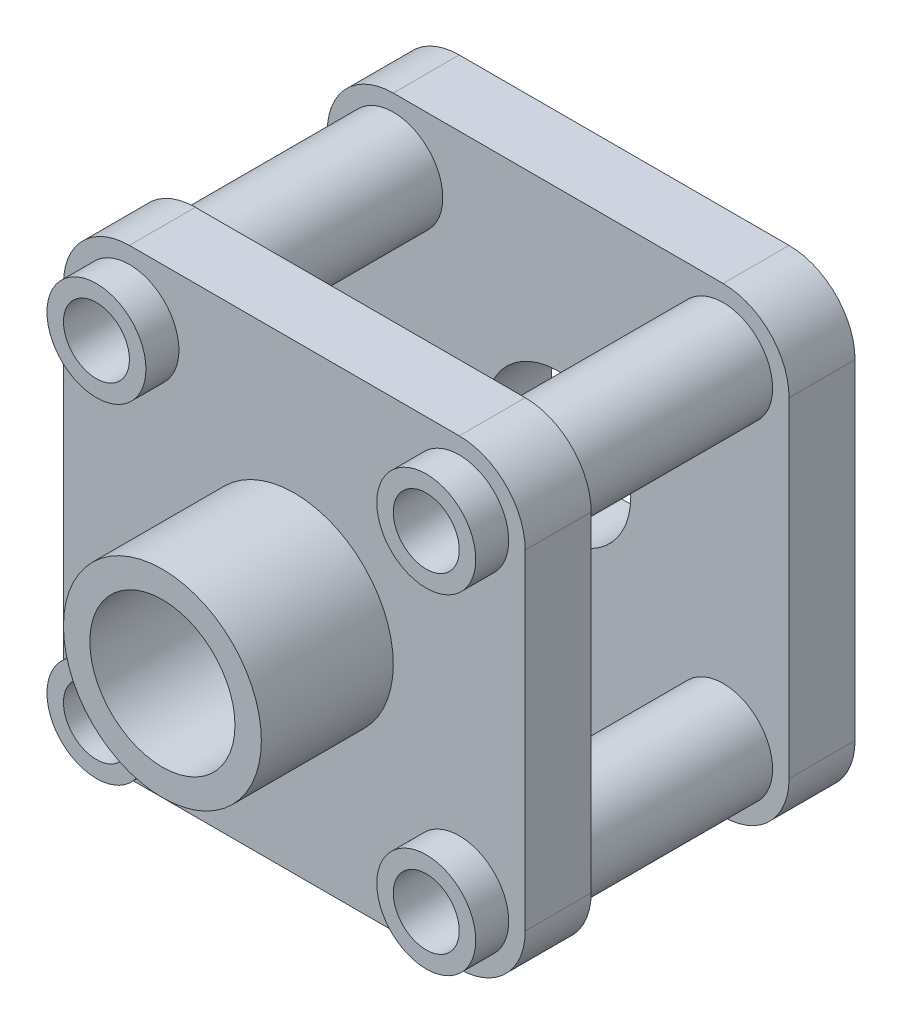
ISO-10303-21;
HEADER;
FILE_DESCRIPTION(('STEP AP214'),'2;1');
FILE_NAME('part.step','',(''),(''),'','','');
FILE_SCHEMA(('AUTOMOTIVE_DESIGN { 1 0 10303 214 1 1 1 1 }'));
ENDSEC;
DATA;
#1=APPLICATION_CONTEXT('core data for automotive mechanical design processes');
#2=APPLICATION_PROTOCOL_DEFINITION('international standard','automotive_design',2000,#1);
#3=PRODUCT_CONTEXT('',#1,'mechanical');
#4=PRODUCT('Part','Part','',(#3));
#5=PRODUCT_RELATED_PRODUCT_CATEGORY('part','',(#4));
#6=PRODUCT_DEFINITION_FORMATION('','',#4);
#7=PRODUCT_DEFINITION_CONTEXT('part definition',#1,'design');
#8=PRODUCT_DEFINITION('design','',#6,#7);
#9=PRODUCT_DEFINITION_SHAPE('','',#8);
#10=(LENGTH_UNIT() NAMED_UNIT(*) SI_UNIT(.MILLI.,.METRE.));
#11=(NAMED_UNIT(*) PLANE_ANGLE_UNIT() SI_UNIT($,.RADIAN.));
#12=(NAMED_UNIT(*) SI_UNIT($,.STERADIAN.) SOLID_ANGLE_UNIT());
#13=UNCERTAINTY_MEASURE_WITH_UNIT(LENGTH_MEASURE(1.E-05),#10,'distance_accuracy_value','');
#14=(GEOMETRIC_REPRESENTATION_CONTEXT(3) GLOBAL_UNCERTAINTY_ASSIGNED_CONTEXT((#13)) GLOBAL_UNIT_ASSIGNED_CONTEXT((#10,
#11,#12)) REPRESENTATION_CONTEXT('',''));
#15=CARTESIAN_POINT('',(0.,0.,0.));
#16=DIRECTION('',(0.,0.,1.));
#17=DIRECTION('',(1.,0.,0.));
#18=AXIS2_PLACEMENT_3D('',#15,#16,#17);
#19=CARTESIAN_POINT('',(0.,70.,10.));
#20=DIRECTION('',(1.,0.,0.));
#21=DIRECTION('',(0.,0.,-1.));
#22=AXIS2_PLACEMENT_3D('',#19,#20,#21);
#23=PLANE('',#22);
#24=DIRECTION('',(0.,-1.,0.));
#25=VECTOR('',#24,1.);
#26=CARTESIAN_POINT('',(0.,70.,0.));
#27=LINE('',#26,#25);
#28=CARTESIAN_POINT('',(0.,60.,0.));
#29=VERTEX_POINT('',#28);
#30=CARTESIAN_POINT('',(0.,10.,0.));
#31=VERTEX_POINT('',#30);
#32=EDGE_CURVE('E216',#29,#31,#27,.T.);
#33=ORIENTED_EDGE('',*,*,#32,.T.);
#34=DIRECTION('',(0.,0.,-1.));
#35=VECTOR('',#34,1.);
#36=CARTESIAN_POINT('',(0.,10.,10.));
#37=LINE('',#36,#35);
#38=CARTESIAN_POINT('',(0.,10.,10.));
#39=VERTEX_POINT('',#38);
#40=EDGE_CURVE('E11',#31,#39,#37,.F.);
#41=ORIENTED_EDGE('',*,*,#40,.T.);
#42=DIRECTION('',(0.,-1.,0.));
#43=VECTOR('',#42,1.);
#44=CARTESIAN_POINT('',(0.,70.,10.));
#45=LINE('',#44,#43);
#46=CARTESIAN_POINT('',(0.,60.,10.));
#47=VERTEX_POINT('',#46);
#48=EDGE_CURVE('E217',#47,#39,#45,.T.);
#49=ORIENTED_EDGE('',*,*,#48,.F.);
#50=DIRECTION('',(0.,0.,-1.));
#51=VECTOR('',#50,1.);
#52=CARTESIAN_POINT('',(0.,60.,10.));
#53=LINE('',#52,#51);
#54=EDGE_CURVE('E52',#47,#29,#53,.T.);
#55=ORIENTED_EDGE('',*,*,#54,.T.);
#56=EDGE_LOOP('',(#33,#41,#49,#55));
#57=FACE_BOUND('',#56,.T.);
#58=ADVANCED_FACE('F44',(#57),#23,.F.);
#59=CARTESIAN_POINT('',(0.,0.,10.));
#60=DIRECTION('',(0.,1.,0.));
#61=DIRECTION('',(0.,0.,1.));
#62=AXIS2_PLACEMENT_3D('',#59,#60,#61);
#63=PLANE('',#62);
#64=DIRECTION('',(1.,0.,0.));
#65=VECTOR('',#64,1.);
#66=CARTESIAN_POINT('',(0.,0.,0.));
#67=LINE('',#66,#65);
#68=CARTESIAN_POINT('',(10.,0.,0.));
#69=VERTEX_POINT('',#68);
#70=CARTESIAN_POINT('',(60.,0.,0.));
#71=VERTEX_POINT('',#70);
#72=EDGE_CURVE('E234',#69,#71,#67,.T.);
#73=ORIENTED_EDGE('',*,*,#72,.T.);
#74=DIRECTION('',(0.,0.,-1.));
#75=VECTOR('',#74,1.);
#76=CARTESIAN_POINT('',(60.,0.,10.));
#77=LINE('',#76,#75);
#78=CARTESIAN_POINT('',(60.,0.,10.));
#79=VERTEX_POINT('',#78);
#80=EDGE_CURVE('E58',#71,#79,#77,.F.);
#81=ORIENTED_EDGE('',*,*,#80,.T.);
#82=DIRECTION('',(1.,0.,0.));
#83=VECTOR('',#82,1.);
#84=CARTESIAN_POINT('',(0.,0.,10.));
#85=LINE('',#84,#83);
#86=CARTESIAN_POINT('',(10.,0.,10.));
#87=VERTEX_POINT('',#86);
#88=EDGE_CURVE('E225',#87,#79,#85,.T.);
#89=ORIENTED_EDGE('',*,*,#88,.F.);
#90=DIRECTION('',(0.,0.,-1.));
#91=VECTOR('',#90,1.);
#92=CARTESIAN_POINT('',(10.,0.,10.));
#93=LINE('',#92,#91);
#94=EDGE_CURVE('E311',#87,#69,#93,.T.);
#95=ORIENTED_EDGE('',*,*,#94,.T.);
#96=EDGE_LOOP('',(#73,#81,#89,#95));
#97=FACE_BOUND('',#96,.T.);
#98=ADVANCED_FACE('F328',(#97),#63,.F.);
#99=CARTESIAN_POINT('',(70.,0.,10.));
#100=DIRECTION('',(-1.,0.,0.));
#101=DIRECTION('',(0.,0.,1.));
#102=AXIS2_PLACEMENT_3D('',#99,#100,#101);
#103=PLANE('',#102);
#104=DIRECTION('',(0.,1.,0.));
#105=VECTOR('',#104,1.);
#106=CARTESIAN_POINT('',(70.,0.,0.));
#107=LINE('',#106,#105);
#108=CARTESIAN_POINT('',(70.,10.,0.));
#109=VERTEX_POINT('',#108);
#110=CARTESIAN_POINT('',(70.,60.,0.));
#111=VERTEX_POINT('',#110);
#112=EDGE_CURVE('E236',#109,#111,#107,.T.);
#113=ORIENTED_EDGE('',*,*,#112,.T.);
#114=DIRECTION('',(0.,0.,-1.));
#115=VECTOR('',#114,1.);
#116=CARTESIAN_POINT('',(70.,60.,10.));
#117=LINE('',#116,#115);
#118=CARTESIAN_POINT('',(70.,60.,10.));
#119=VERTEX_POINT('',#118);
#120=EDGE_CURVE('E305',#111,#119,#117,.F.);
#121=ORIENTED_EDGE('',*,*,#120,.T.);
#122=DIRECTION('',(0.,1.,0.));
#123=VECTOR('',#122,1.);
#124=CARTESIAN_POINT('',(70.,0.,10.));
#125=LINE('',#124,#123);
#126=CARTESIAN_POINT('',(70.,10.,10.));
#127=VERTEX_POINT('',#126);
#128=EDGE_CURVE('E224',#127,#119,#125,.T.);
#129=ORIENTED_EDGE('',*,*,#128,.F.);
#130=DIRECTION('',(0.,0.,-1.));
#131=VECTOR('',#130,1.);
#132=CARTESIAN_POINT('',(70.,10.,10.));
#133=LINE('',#132,#131);
#134=EDGE_CURVE('E299',#127,#109,#133,.T.);
#135=ORIENTED_EDGE('',*,*,#134,.T.);
#136=EDGE_LOOP('',(#113,#121,#129,#135));
#137=FACE_BOUND('',#136,.T.);
#138=ADVANCED_FACE('F336',(#137),#103,.F.);
#139=CARTESIAN_POINT('',(70.,70.,10.));
#140=DIRECTION('',(0.,-1.,0.));
#141=DIRECTION('',(0.,0.,-1.));
#142=AXIS2_PLACEMENT_3D('',#139,#140,#141);
#143=PLANE('',#142);
#144=DIRECTION('',(-1.,0.,0.));
#145=VECTOR('',#144,1.);
#146=CARTESIAN_POINT('',(70.,70.,10.));
#147=LINE('',#146,#145);
#148=CARTESIAN_POINT('',(60.,70.,10.));
#149=VERTEX_POINT('',#148);
#150=CARTESIAN_POINT('',(10.,70.,10.));
#151=VERTEX_POINT('',#150);
#152=EDGE_CURVE('E226',#149,#151,#147,.T.);
#153=ORIENTED_EDGE('',*,*,#152,.F.);
#154=DIRECTION('',(0.,0.,-1.));
#155=VECTOR('',#154,1.);
#156=CARTESIAN_POINT('',(60.,70.,10.));
#157=LINE('',#156,#155);
#158=CARTESIAN_POINT('',(60.,70.,0.));
#159=VERTEX_POINT('',#158);
#160=EDGE_CURVE('E287',#149,#159,#157,.T.);
#161=ORIENTED_EDGE('',*,*,#160,.T.);
#162=DIRECTION('',(-1.,0.,0.));
#163=VECTOR('',#162,1.);
#164=CARTESIAN_POINT('',(70.,70.,0.));
#165=LINE('',#164,#163);
#166=CARTESIAN_POINT('',(10.,70.,0.));
#167=VERTEX_POINT('',#166);
#168=EDGE_CURVE('E222',#159,#167,#165,.T.);
#169=ORIENTED_EDGE('',*,*,#168,.T.);
#170=DIRECTION('',(0.,0.,-1.));
#171=VECTOR('',#170,1.);
#172=CARTESIAN_POINT('',(10.,70.,10.));
#173=LINE('',#172,#171);
#174=EDGE_CURVE('E286',#167,#151,#173,.F.);
#175=ORIENTED_EDGE('',*,*,#174,.T.);
#176=EDGE_LOOP('',(#153,#161,#169,#175));
#177=FACE_BOUND('',#176,.T.);
#178=ADVANCED_FACE('F349',(#177),#143,.F.);
#179=CARTESIAN_POINT('',(0.,0.,10.));
#180=DIRECTION('',(0.,0.,1.));
#181=DIRECTION('',(1.,0.,0.));
#182=AXIS2_PLACEMENT_3D('',#179,#180,#181);
#183=PLANE('',#182);
#184=CARTESIAN_POINT('',(35.,35.,10.));
#185=DIRECTION('',(0.,0.,1.));
#186=DIRECTION('',(1.,0.,0.));
#187=AXIS2_PLACEMENT_3D('',#184,#185,#186);
#188=CIRCLE('',#187,11.);
#189=CARTESIAN_POINT('',(46.,35.,10.));
#190=VERTEX_POINT('',#189);
#191=EDGE_CURVE('E260',#190,#190,#188,.T.);
#192=ORIENTED_EDGE('',*,*,#191,.F.);
#193=EDGE_LOOP('',(#192));
#194=FACE_BOUND('',#193,.T.);
#195=CARTESIAN_POINT('',(10.,60.,10.));
#196=DIRECTION('',(0.,0.,1.));
#197=DIRECTION('',(1.,0.,0.));
#198=AXIS2_PLACEMENT_3D('',#195,#196,#197);
#199=CIRCLE('',#198,7.5);
#200=CARTESIAN_POINT('',(17.5,60.,10.));
#201=VERTEX_POINT('',#200);
#202=EDGE_CURVE('E198',#201,#201,#199,.T.);
#203=ORIENTED_EDGE('',*,*,#202,.F.);
#204=EDGE_LOOP('',(#203));
#205=FACE_BOUND('',#204,.T.);
#206=CARTESIAN_POINT('',(60.,60.,10.));
#207=DIRECTION('',(0.,0.,1.));
#208=DIRECTION('',(1.,0.,0.));
#209=AXIS2_PLACEMENT_3D('',#206,#207,#208);
#210=CIRCLE('',#209,7.49999999999999);
#211=CARTESIAN_POINT('',(67.5,60.,10.));
#212=VERTEX_POINT('',#211);
#213=EDGE_CURVE('E200',#212,#212,#210,.T.);
#214=ORIENTED_EDGE('',*,*,#213,.F.);
#215=EDGE_LOOP('',(#214));
#216=FACE_BOUND('',#215,.T.);
#217=CARTESIAN_POINT('',(60.,10.,10.));
#218=DIRECTION('',(0.,0.,1.));
#219=DIRECTION('',(1.,0.,0.));
#220=AXIS2_PLACEMENT_3D('',#217,#218,#219);
#221=CIRCLE('',#220,7.50000000000001);
#222=CARTESIAN_POINT('',(67.5,10.,10.));
#223=VERTEX_POINT('',#222);
#224=EDGE_CURVE('E204',#223,#223,#221,.T.);
#225=ORIENTED_EDGE('',*,*,#224,.F.);
#226=EDGE_LOOP('',(#225));
#227=FACE_BOUND('',#226,.T.);
#228=CARTESIAN_POINT('',(10.,10.,10.));
#229=DIRECTION('',(0.,0.,1.));
#230=DIRECTION('',(1.,0.,0.));
#231=AXIS2_PLACEMENT_3D('',#228,#229,#230);
#232=CIRCLE('',#231,7.5);
#233=CARTESIAN_POINT('',(17.5,10.,10.));
#234=VERTEX_POINT('',#233);
#235=EDGE_CURVE('E214',#234,#234,#232,.T.);
#236=ORIENTED_EDGE('',*,*,#235,.F.);
#237=EDGE_LOOP('',(#236));
#238=FACE_BOUND('',#237,.T.);
#239=ORIENTED_EDGE('',*,*,#128,.T.);
#240=CARTESIAN_POINT('',(60.,60.,10.));
#241=DIRECTION('',(0.,0.,1.));
#242=DIRECTION('',(1.,0.,0.));
#243=AXIS2_PLACEMENT_3D('',#240,#241,#242);
#244=CIRCLE('',#243,10.);
#245=EDGE_CURVE('E307',#119,#149,#244,.T.);
#246=ORIENTED_EDGE('',*,*,#245,.T.);
#247=ORIENTED_EDGE('',*,*,#152,.T.);
#248=CARTESIAN_POINT('',(10.,60.,10.));
#249=DIRECTION('',(0.,0.,1.));
#250=DIRECTION('',(1.,0.,0.));
#251=AXIS2_PLACEMENT_3D('',#248,#249,#250);
#252=CIRCLE('',#251,10.);
#253=EDGE_CURVE('E302',#151,#47,#252,.T.);
#254=ORIENTED_EDGE('',*,*,#253,.T.);
#255=ORIENTED_EDGE('',*,*,#48,.T.);
#256=CARTESIAN_POINT('',(10.,10.,10.));
#257=DIRECTION('',(0.,0.,1.));
#258=DIRECTION('',(1.,0.,0.));
#259=AXIS2_PLACEMENT_3D('',#256,#257,#258);
#260=CIRCLE('',#259,10.);
#261=EDGE_CURVE('E66',#39,#87,#260,.T.);
#262=ORIENTED_EDGE('',*,*,#261,.T.);
#263=ORIENTED_EDGE('',*,*,#88,.T.);
#264=CARTESIAN_POINT('',(60.,10.,10.));
#265=DIRECTION('',(0.,0.,1.));
#266=DIRECTION('',(1.,0.,0.));
#267=AXIS2_PLACEMENT_3D('',#264,#265,#266);
#268=CIRCLE('',#267,10.);
#269=EDGE_CURVE('E310',#79,#127,#268,.T.);
#270=ORIENTED_EDGE('',*,*,#269,.T.);
#271=EDGE_LOOP('',(#239,#246,#247,#254,#255,#262,#263,#270));
#272=FACE_BOUND('',#271,.T.);
#273=ADVANCED_FACE('F331',(#194,#205,#216,#227,#238,#272),#183,.T.);
#274=CARTESIAN_POINT('',(0.,0.,0.));
#275=DIRECTION('',(0.,0.,1.));
#276=DIRECTION('',(1.,0.,0.));
#277=AXIS2_PLACEMENT_3D('',#274,#275,#276);
#278=PLANE('',#277);
#279=CARTESIAN_POINT('',(10.,60.,0.));
#280=DIRECTION('',(0.,0.,1.));
#281=DIRECTION('',(1.,0.,0.));
#282=AXIS2_PLACEMENT_3D('',#279,#280,#281);
#283=CIRCLE('',#282,5.);
#284=CARTESIAN_POINT('',(15.,60.,0.));
#285=VERTEX_POINT('',#284);
#286=EDGE_CURVE('E984',#285,#285,#283,.T.);
#287=ORIENTED_EDGE('',*,*,#286,.T.);
#288=EDGE_LOOP('',(#287));
#289=FACE_BOUND('',#288,.T.);
#290=CARTESIAN_POINT('',(60.,10.,0.));
#291=DIRECTION('',(0.,0.,1.));
#292=DIRECTION('',(1.,0.,0.));
#293=AXIS2_PLACEMENT_3D('',#290,#291,#292);
#294=CIRCLE('',#293,5.);
#295=CARTESIAN_POINT('',(65.,10.,0.));
#296=VERTEX_POINT('',#295);
#297=EDGE_CURVE('E990',#296,#296,#294,.T.);
#298=ORIENTED_EDGE('',*,*,#297,.T.);
#299=EDGE_LOOP('',(#298));
#300=FACE_BOUND('',#299,.T.);
#301=CARTESIAN_POINT('',(9.99999999999999,10.,0.));
#302=DIRECTION('',(0.,0.,1.));
#303=DIRECTION('',(1.,0.,0.));
#304=AXIS2_PLACEMENT_3D('',#301,#302,#303);
#305=CIRCLE('',#304,5.);
#306=CARTESIAN_POINT('',(15.,10.,0.));
#307=VERTEX_POINT('',#306);
#308=EDGE_CURVE('E994',#307,#307,#305,.T.);
#309=ORIENTED_EDGE('',*,*,#308,.T.);
#310=EDGE_LOOP('',(#309));
#311=FACE_BOUND('',#310,.T.);
#312=CARTESIAN_POINT('',(60.,60.,0.));
#313=DIRECTION('',(0.,0.,1.));
#314=DIRECTION('',(1.,0.,0.));
#315=AXIS2_PLACEMENT_3D('',#312,#313,#314);
#316=CIRCLE('',#315,5.);
#317=CARTESIAN_POINT('',(65.,60.,0.));
#318=VERTEX_POINT('',#317);
#319=EDGE_CURVE('E987',#318,#318,#316,.T.);
#320=ORIENTED_EDGE('',*,*,#319,.T.);
#321=EDGE_LOOP('',(#320));
#322=FACE_BOUND('',#321,.T.);
#323=CARTESIAN_POINT('',(35.,35.,0.));
#324=DIRECTION('',(0.,0.,1.));
#325=DIRECTION('',(1.,0.,0.));
#326=AXIS2_PLACEMENT_3D('',#323,#324,#325);
#327=CIRCLE('',#326,11.);
#328=CARTESIAN_POINT('',(46.,35.,0.));
#329=VERTEX_POINT('',#328);
#330=EDGE_CURVE('E258',#329,#329,#327,.T.);
#331=ORIENTED_EDGE('',*,*,#330,.T.);
#332=EDGE_LOOP('',(#331));
#333=FACE_BOUND('',#332,.T.);
#334=ORIENTED_EDGE('',*,*,#168,.F.);
#335=CARTESIAN_POINT('',(60.,60.,0.));
#336=DIRECTION('',(0.,0.,1.));
#337=DIRECTION('',(1.,0.,0.));
#338=AXIS2_PLACEMENT_3D('',#335,#336,#337);
#339=CIRCLE('',#338,10.);
#340=EDGE_CURVE('E300',#159,#111,#339,.F.);
#341=ORIENTED_EDGE('',*,*,#340,.T.);
#342=ORIENTED_EDGE('',*,*,#112,.F.);
#343=CARTESIAN_POINT('',(60.,10.,0.));
#344=DIRECTION('',(0.,0.,1.));
#345=DIRECTION('',(1.,0.,0.));
#346=AXIS2_PLACEMENT_3D('',#343,#344,#345);
#347=CIRCLE('',#346,10.);
#348=EDGE_CURVE('E294',#109,#71,#347,.F.);
#349=ORIENTED_EDGE('',*,*,#348,.T.);
#350=ORIENTED_EDGE('',*,*,#72,.F.);
#351=CARTESIAN_POINT('',(10.,10.,0.));
#352=DIRECTION('',(0.,0.,1.));
#353=DIRECTION('',(1.,0.,0.));
#354=AXIS2_PLACEMENT_3D('',#351,#352,#353);
#355=CIRCLE('',#354,10.);
#356=EDGE_CURVE('E291',#69,#31,#355,.F.);
#357=ORIENTED_EDGE('',*,*,#356,.T.);
#358=ORIENTED_EDGE('',*,*,#32,.F.);
#359=CARTESIAN_POINT('',(10.,60.,0.));
#360=DIRECTION('',(0.,0.,1.));
#361=DIRECTION('',(1.,0.,0.));
#362=AXIS2_PLACEMENT_3D('',#359,#360,#361);
#363=CIRCLE('',#362,10.);
#364=EDGE_CURVE('E293',#29,#167,#363,.F.);
#365=ORIENTED_EDGE('',*,*,#364,.T.);
#366=EDGE_LOOP('',(#334,#341,#342,#349,#350,#357,#358,#365));
#367=FACE_BOUND('',#366,.T.);
#368=ADVANCED_FACE('F323',(#289,#300,#311,#322,#333,#367),#278,.F.);
#369=CARTESIAN_POINT('',(10.,10.,40.));
#370=DIRECTION('',(0.,0.,-1.));
#371=DIRECTION('',(-1.,0.,0.));
#372=AXIS2_PLACEMENT_3D('',#369,#370,#371);
#373=CYLINDRICAL_SURFACE('',#372,7.5);
#374=CARTESIAN_POINT('',(10.,10.,40.));
#375=DIRECTION('',(0.,0.,1.));
#376=DIRECTION('',(1.,0.,0.));
#377=AXIS2_PLACEMENT_3D('',#374,#375,#376);
#378=CIRCLE('',#377,7.5);
#379=CARTESIAN_POINT('',(17.5,10.,40.));
#380=VERTEX_POINT('',#379);
#381=EDGE_CURVE('E213',#380,#380,#378,.T.);
#382=ORIENTED_EDGE('',*,*,#381,.F.);
#383=EDGE_LOOP('',(#382));
#384=FACE_BOUND('',#383,.T.);
#385=ORIENTED_EDGE('',*,*,#235,.T.);
#386=EDGE_LOOP('',(#385));
#387=FACE_BOUND('',#386,.T.);
#388=ADVANCED_FACE('F659',(#384,#387),#373,.T.);
#389=CARTESIAN_POINT('',(60.,10.,40.));
#390=DIRECTION('',(0.,0.,-1.));
#391=DIRECTION('',(-1.,0.,0.));
#392=AXIS2_PLACEMENT_3D('',#389,#390,#391);
#393=CYLINDRICAL_SURFACE('',#392,7.50000000000001);
#394=CARTESIAN_POINT('',(60.,10.,40.));
#395=DIRECTION('',(0.,0.,1.));
#396=DIRECTION('',(1.,0.,0.));
#397=AXIS2_PLACEMENT_3D('',#394,#395,#396);
#398=CIRCLE('',#397,7.50000000000001);
#399=CARTESIAN_POINT('',(67.5,10.,40.));
#400=VERTEX_POINT('',#399);
#401=EDGE_CURVE('E206',#400,#400,#398,.T.);
#402=ORIENTED_EDGE('',*,*,#401,.F.);
#403=EDGE_LOOP('',(#402));
#404=FACE_BOUND('',#403,.T.);
#405=ORIENTED_EDGE('',*,*,#224,.T.);
#406=EDGE_LOOP('',(#405));
#407=FACE_BOUND('',#406,.T.);
#408=ADVANCED_FACE('F647',(#404,#407),#393,.T.);
#409=CARTESIAN_POINT('',(60.,60.,40.));
#410=DIRECTION('',(0.,0.,-1.));
#411=DIRECTION('',(-1.,0.,0.));
#412=AXIS2_PLACEMENT_3D('',#409,#410,#411);
#413=CYLINDRICAL_SURFACE('',#412,7.49999999999999);
#414=CARTESIAN_POINT('',(60.,60.,40.));
#415=DIRECTION('',(0.,0.,1.));
#416=DIRECTION('',(1.,0.,0.));
#417=AXIS2_PLACEMENT_3D('',#414,#415,#416);
#418=CIRCLE('',#417,7.49999999999999);
#419=CARTESIAN_POINT('',(67.5,60.,40.));
#420=VERTEX_POINT('',#419);
#421=EDGE_CURVE('E205',#420,#420,#418,.T.);
#422=ORIENTED_EDGE('',*,*,#421,.F.);
#423=EDGE_LOOP('',(#422));
#424=FACE_BOUND('',#423,.T.);
#425=ORIENTED_EDGE('',*,*,#213,.T.);
#426=EDGE_LOOP('',(#425));
#427=FACE_BOUND('',#426,.T.);
#428=ADVANCED_FACE('F639',(#424,#427),#413,.T.);
#429=CARTESIAN_POINT('',(10.,60.,40.));
#430=DIRECTION('',(0.,0.,-1.));
#431=DIRECTION('',(-1.,0.,0.));
#432=AXIS2_PLACEMENT_3D('',#429,#430,#431);
#433=CYLINDRICAL_SURFACE('',#432,7.5);
#434=CARTESIAN_POINT('',(10.,60.,40.));
#435=DIRECTION('',(0.,0.,1.));
#436=DIRECTION('',(1.,0.,0.));
#437=AXIS2_PLACEMENT_3D('',#434,#435,#436);
#438=CIRCLE('',#437,7.5);
#439=CARTESIAN_POINT('',(17.5,60.,40.));
#440=VERTEX_POINT('',#439);
#441=EDGE_CURVE('E192',#440,#440,#438,.T.);
#442=ORIENTED_EDGE('',*,*,#441,.F.);
#443=EDGE_LOOP('',(#442));
#444=FACE_BOUND('',#443,.T.);
#445=ORIENTED_EDGE('',*,*,#202,.T.);
#446=EDGE_LOOP('',(#445));
#447=FACE_BOUND('',#446,.T.);
#448=ADVANCED_FACE('F629',(#444,#447),#433,.T.);
#449=CARTESIAN_POINT('',(0.,0.,50.));
#450=DIRECTION('',(1.,0.,0.));
#451=DIRECTION('',(0.,0.,-1.));
#452=AXIS2_PLACEMENT_3D('',#449,#450,#451);
#453=PLANE('',#452);
#454=DIRECTION('',(0.,-1.,0.));
#455=VECTOR('',#454,1.);
#456=CARTESIAN_POINT('',(0.,0.,50.));
#457=LINE('',#456,#455);
#458=CARTESIAN_POINT('',(0.,60.,50.));
#459=VERTEX_POINT('',#458);
#460=CARTESIAN_POINT('',(0.,10.,50.));
#461=VERTEX_POINT('',#460);
#462=EDGE_CURVE('E184',#459,#461,#457,.T.);
#463=ORIENTED_EDGE('',*,*,#462,.F.);
#464=DIRECTION('',(0.,0.,-1.));
#465=VECTOR('',#464,1.);
#466=CARTESIAN_POINT('',(0.,60.,50.));
#467=LINE('',#466,#465);
#468=CARTESIAN_POINT('',(0.,60.,40.));
#469=VERTEX_POINT('',#468);
#470=EDGE_CURVE('E280',#459,#469,#467,.T.);
#471=ORIENTED_EDGE('',*,*,#470,.T.);
#472=DIRECTION('',(0.,-1.,0.));
#473=VECTOR('',#472,1.);
#474=CARTESIAN_POINT('',(0.,0.,40.));
#475=LINE('',#474,#473);
#476=CARTESIAN_POINT('',(0.,10.,40.));
#477=VERTEX_POINT('',#476);
#478=EDGE_CURVE('E953',#469,#477,#475,.T.);
#479=ORIENTED_EDGE('',*,*,#478,.T.);
#480=DIRECTION('',(0.,0.,-1.));
#481=VECTOR('',#480,1.);
#482=CARTESIAN_POINT('',(0.,10.,50.));
#483=LINE('',#482,#481);
#484=EDGE_CURVE('E279',#477,#461,#483,.F.);
#485=ORIENTED_EDGE('',*,*,#484,.T.);
#486=EDGE_LOOP('',(#463,#471,#479,#485));
#487=FACE_BOUND('',#486,.T.);
#488=ADVANCED_FACE('F619',(#487),#453,.F.);
#489=CARTESIAN_POINT('',(70.,0.,50.));
#490=DIRECTION('',(0.,1.,0.));
#491=DIRECTION('',(0.,0.,1.));
#492=AXIS2_PLACEMENT_3D('',#489,#490,#491);
#493=PLANE('',#492);
#494=DIRECTION('',(1.,0.,0.));
#495=VECTOR('',#494,1.);
#496=CARTESIAN_POINT('',(70.,0.,50.));
#497=LINE('',#496,#495);
#498=CARTESIAN_POINT('',(10.,0.,50.));
#499=VERTEX_POINT('',#498);
#500=CARTESIAN_POINT('',(60.,0.,50.));
#501=VERTEX_POINT('',#500);
#502=EDGE_CURVE('E186',#499,#501,#497,.T.);
#503=ORIENTED_EDGE('',*,*,#502,.F.);
#504=DIRECTION('',(0.,0.,-1.));
#505=VECTOR('',#504,1.);
#506=CARTESIAN_POINT('',(10.,0.,50.));
#507=LINE('',#506,#505);
#508=CARTESIAN_POINT('',(10.,0.,40.));
#509=VERTEX_POINT('',#508);
#510=EDGE_CURVE('E285',#499,#509,#507,.T.);
#511=ORIENTED_EDGE('',*,*,#510,.T.);
#512=DIRECTION('',(1.,0.,0.));
#513=VECTOR('',#512,1.);
#514=CARTESIAN_POINT('',(70.,0.,40.));
#515=LINE('',#514,#513);
#516=CARTESIAN_POINT('',(60.,0.,40.));
#517=VERTEX_POINT('',#516);
#518=EDGE_CURVE('E194',#509,#517,#515,.T.);
#519=ORIENTED_EDGE('',*,*,#518,.T.);
#520=DIRECTION('',(0.,0.,-1.));
#521=VECTOR('',#520,1.);
#522=CARTESIAN_POINT('',(60.,0.,50.));
#523=LINE('',#522,#521);
#524=EDGE_CURVE('E284',#517,#501,#523,.F.);
#525=ORIENTED_EDGE('',*,*,#524,.T.);
#526=EDGE_LOOP('',(#503,#511,#519,#525));
#527=FACE_BOUND('',#526,.T.);
#528=ADVANCED_FACE('F607',(#527),#493,.F.);
#529=CARTESIAN_POINT('',(70.,70.,50.));
#530=DIRECTION('',(-1.,0.,0.));
#531=DIRECTION('',(0.,0.,1.));
#532=AXIS2_PLACEMENT_3D('',#529,#530,#531);
#533=PLANE('',#532);
#534=DIRECTION('',(0.,1.,0.));
#535=VECTOR('',#534,1.);
#536=CARTESIAN_POINT('',(70.,70.,40.));
#537=LINE('',#536,#535);
#538=CARTESIAN_POINT('',(70.,10.,40.));
#539=VERTEX_POINT('',#538);
#540=CARTESIAN_POINT('',(70.,60.,40.));
#541=VERTEX_POINT('',#540);
#542=EDGE_CURVE('E187',#539,#541,#537,.T.);
#543=ORIENTED_EDGE('',*,*,#542,.T.);
#544=DIRECTION('',(0.,0.,-1.));
#545=VECTOR('',#544,1.);
#546=CARTESIAN_POINT('',(70.,60.,50.));
#547=LINE('',#546,#545);
#548=CARTESIAN_POINT('',(70.,60.,50.));
#549=VERTEX_POINT('',#548);
#550=EDGE_CURVE('E165',#541,#549,#547,.F.);
#551=ORIENTED_EDGE('',*,*,#550,.T.);
#552=DIRECTION('',(0.,1.,0.));
#553=VECTOR('',#552,1.);
#554=CARTESIAN_POINT('',(70.,70.,50.));
#555=LINE('',#554,#553);
#556=CARTESIAN_POINT('',(70.,10.,50.));
#557=VERTEX_POINT('',#556);
#558=EDGE_CURVE('E960',#557,#549,#555,.T.);
#559=ORIENTED_EDGE('',*,*,#558,.F.);
#560=DIRECTION('',(0.,0.,-1.));
#561=VECTOR('',#560,1.);
#562=CARTESIAN_POINT('',(70.,10.,50.));
#563=LINE('',#562,#561);
#564=EDGE_CURVE('E169',#557,#539,#563,.T.);
#565=ORIENTED_EDGE('',*,*,#564,.T.);
#566=EDGE_LOOP('',(#543,#551,#559,#565));
#567=FACE_BOUND('',#566,.T.);
#568=ADVANCED_FACE('F604',(#567),#533,.F.);
#569=CARTESIAN_POINT('',(0.,70.,50.));
#570=DIRECTION('',(0.,-1.,0.));
#571=DIRECTION('',(0.,0.,-1.));
#572=AXIS2_PLACEMENT_3D('',#569,#570,#571);
#573=PLANE('',#572);
#574=DIRECTION('',(-1.,0.,0.));
#575=VECTOR('',#574,1.);
#576=CARTESIAN_POINT('',(0.,70.,50.));
#577=LINE('',#576,#575);
#578=CARTESIAN_POINT('',(60.,70.,50.));
#579=VERTEX_POINT('',#578);
#580=CARTESIAN_POINT('',(10.,70.,50.));
#581=VERTEX_POINT('',#580);
#582=EDGE_CURVE('E177',#579,#581,#577,.T.);
#583=ORIENTED_EDGE('',*,*,#582,.F.);
#584=DIRECTION('',(0.,0.,-1.));
#585=VECTOR('',#584,1.);
#586=CARTESIAN_POINT('',(60.,70.,50.));
#587=LINE('',#586,#585);
#588=CARTESIAN_POINT('',(60.,70.,40.));
#589=VERTEX_POINT('',#588);
#590=EDGE_CURVE('E161',#579,#589,#587,.T.);
#591=ORIENTED_EDGE('',*,*,#590,.T.);
#592=DIRECTION('',(-1.,0.,0.));
#593=VECTOR('',#592,1.);
#594=CARTESIAN_POINT('',(0.,70.,40.));
#595=LINE('',#594,#593);
#596=CARTESIAN_POINT('',(10.,70.,40.));
#597=VERTEX_POINT('',#596);
#598=EDGE_CURVE('E176',#589,#597,#595,.T.);
#599=ORIENTED_EDGE('',*,*,#598,.T.);
#600=DIRECTION('',(0.,0.,-1.));
#601=VECTOR('',#600,1.);
#602=CARTESIAN_POINT('',(10.,70.,50.));
#603=LINE('',#602,#601);
#604=EDGE_CURVE('E181',#597,#581,#603,.F.);
#605=ORIENTED_EDGE('',*,*,#604,.T.);
#606=EDGE_LOOP('',(#583,#591,#599,#605));
#607=FACE_BOUND('',#606,.T.);
#608=ADVANCED_FACE('F174',(#607),#573,.F.);
#609=CARTESIAN_POINT('',(0.,0.,50.));
#610=DIRECTION('',(0.,0.,-1.));
#611=DIRECTION('',(-1.,0.,0.));
#612=AXIS2_PLACEMENT_3D('',#609,#610,#611);
#613=PLANE('',#612);
#614=CARTESIAN_POINT('',(35.,35.,50.));
#615=DIRECTION('',(0.,0.,-1.));
#616=DIRECTION('',(-1.,0.,0.));
#617=AXIS2_PLACEMENT_3D('',#614,#615,#616);
#618=CIRCLE('',#617,15.);
#619=CARTESIAN_POINT('',(20.,35.,50.));
#620=VERTEX_POINT('',#619);
#621=EDGE_CURVE('E255',#620,#620,#618,.F.);
#622=ORIENTED_EDGE('',*,*,#621,.F.);
#623=EDGE_LOOP('',(#622));
#624=FACE_BOUND('',#623,.T.);
#625=CARTESIAN_POINT('',(60.,10.,50.));
#626=DIRECTION('',(0.,0.,-1.));
#627=DIRECTION('',(-1.,0.,0.));
#628=AXIS2_PLACEMENT_3D('',#625,#626,#627);
#629=CIRCLE('',#628,7.50000000000001);
#630=CARTESIAN_POINT('',(52.5,10.,50.));
#631=VERTEX_POINT('',#630);
#632=EDGE_CURVE('E248',#631,#631,#629,.F.);
#633=ORIENTED_EDGE('',*,*,#632,.F.);
#634=EDGE_LOOP('',(#633));
#635=FACE_BOUND('',#634,.T.);
#636=CARTESIAN_POINT('',(9.99999999999999,10.,50.));
#637=DIRECTION('',(0.,0.,-1.));
#638=DIRECTION('',(-1.,0.,0.));
#639=AXIS2_PLACEMENT_3D('',#636,#637,#638);
#640=CIRCLE('',#639,7.5);
#641=CARTESIAN_POINT('',(2.5,10.,50.));
#642=VERTEX_POINT('',#641);
#643=EDGE_CURVE('E246',#642,#642,#640,.F.);
#644=ORIENTED_EDGE('',*,*,#643,.F.);
#645=EDGE_LOOP('',(#644));
#646=FACE_BOUND('',#645,.T.);
#647=CARTESIAN_POINT('',(60.,60.,50.));
#648=DIRECTION('',(0.,0.,-1.));
#649=DIRECTION('',(-1.,0.,0.));
#650=AXIS2_PLACEMENT_3D('',#647,#648,#649);
#651=CIRCLE('',#650,7.50000000000001);
#652=CARTESIAN_POINT('',(52.5,60.,50.));
#653=VERTEX_POINT('',#652);
#654=EDGE_CURVE('E243',#653,#653,#651,.F.);
#655=ORIENTED_EDGE('',*,*,#654,.F.);
#656=EDGE_LOOP('',(#655));
#657=FACE_BOUND('',#656,.T.);
#658=CARTESIAN_POINT('',(10.,60.,50.));
#659=DIRECTION('',(0.,0.,-1.));
#660=DIRECTION('',(-1.,0.,0.));
#661=AXIS2_PLACEMENT_3D('',#658,#659,#660);
#662=CIRCLE('',#661,7.5);
#663=CARTESIAN_POINT('',(2.5,60.,50.));
#664=VERTEX_POINT('',#663);
#665=EDGE_CURVE('E233',#664,#664,#662,.F.);
#666=ORIENTED_EDGE('',*,*,#665,.F.);
#667=EDGE_LOOP('',(#666));
#668=FACE_BOUND('',#667,.T.);
#669=ORIENTED_EDGE('',*,*,#558,.T.);
#670=CARTESIAN_POINT('',(60.,60.,50.));
#671=DIRECTION('',(0.,0.,-1.));
#672=DIRECTION('',(-1.,0.,0.));
#673=AXIS2_PLACEMENT_3D('',#670,#671,#672);
#674=CIRCLE('',#673,10.);
#675=EDGE_CURVE('E274',#549,#579,#674,.F.);
#676=ORIENTED_EDGE('',*,*,#675,.T.);
#677=ORIENTED_EDGE('',*,*,#582,.T.);
#678=CARTESIAN_POINT('',(10.,60.,50.));
#679=DIRECTION('',(0.,0.,-1.));
#680=DIRECTION('',(-1.,0.,0.));
#681=AXIS2_PLACEMENT_3D('',#678,#679,#680);
#682=CIRCLE('',#681,10.);
#683=EDGE_CURVE('E275',#581,#459,#682,.F.);
#684=ORIENTED_EDGE('',*,*,#683,.T.);
#685=ORIENTED_EDGE('',*,*,#462,.T.);
#686=CARTESIAN_POINT('',(10.,10.,50.));
#687=DIRECTION('',(0.,0.,-1.));
#688=DIRECTION('',(-1.,0.,0.));
#689=AXIS2_PLACEMENT_3D('',#686,#687,#688);
#690=CIRCLE('',#689,10.);
#691=EDGE_CURVE('E269',#461,#499,#690,.F.);
#692=ORIENTED_EDGE('',*,*,#691,.T.);
#693=ORIENTED_EDGE('',*,*,#502,.T.);
#694=CARTESIAN_POINT('',(60.,10.,50.));
#695=DIRECTION('',(0.,0.,-1.));
#696=DIRECTION('',(-1.,0.,0.));
#697=AXIS2_PLACEMENT_3D('',#694,#695,#696);
#698=CIRCLE('',#697,10.);
#699=EDGE_CURVE('E267',#501,#557,#698,.F.);
#700=ORIENTED_EDGE('',*,*,#699,.T.);
#701=EDGE_LOOP('',(#669,#676,#677,#684,#685,#692,#693,#700));
#702=FACE_BOUND('',#701,.T.);
#703=ADVANCED_FACE('F585',(#624,#635,#646,#657,#668,#702),#613,.F.);
#704=CARTESIAN_POINT('',(0.,0.,40.));
#705=DIRECTION('',(0.,0.,-1.));
#706=DIRECTION('',(-1.,0.,0.));
#707=AXIS2_PLACEMENT_3D('',#704,#705,#706);
#708=PLANE('',#707);
#709=CARTESIAN_POINT('',(35.,35.,40.));
#710=DIRECTION('',(0.,0.,-1.));
#711=DIRECTION('',(-1.,0.,0.));
#712=AXIS2_PLACEMENT_3D('',#709,#710,#711);
#713=CIRCLE('',#712,11.);
#714=CARTESIAN_POINT('',(24.,35.,40.));
#715=VERTEX_POINT('',#714);
#716=EDGE_CURVE('E253',#715,#715,#713,.T.);
#717=ORIENTED_EDGE('',*,*,#716,.F.);
#718=EDGE_LOOP('',(#717));
#719=FACE_BOUND('',#718,.T.);
#720=ORIENTED_EDGE('',*,*,#381,.T.);
#721=EDGE_LOOP('',(#720));
#722=FACE_BOUND('',#721,.T.);
#723=ORIENTED_EDGE('',*,*,#401,.T.);
#724=EDGE_LOOP('',(#723));
#725=FACE_BOUND('',#724,.T.);
#726=ORIENTED_EDGE('',*,*,#421,.T.);
#727=EDGE_LOOP('',(#726));
#728=FACE_BOUND('',#727,.T.);
#729=ORIENTED_EDGE('',*,*,#441,.T.);
#730=EDGE_LOOP('',(#729));
#731=FACE_BOUND('',#730,.T.);
#732=ORIENTED_EDGE('',*,*,#598,.F.);
#733=CARTESIAN_POINT('',(60.,60.,40.));
#734=DIRECTION('',(0.,0.,-1.));
#735=DIRECTION('',(-1.,0.,0.));
#736=AXIS2_PLACEMENT_3D('',#733,#734,#735);
#737=CIRCLE('',#736,10.);
#738=EDGE_CURVE('E158',#589,#541,#737,.T.);
#739=ORIENTED_EDGE('',*,*,#738,.T.);
#740=ORIENTED_EDGE('',*,*,#542,.F.);
#741=CARTESIAN_POINT('',(60.,10.,40.));
#742=DIRECTION('',(0.,0.,-1.));
#743=DIRECTION('',(-1.,0.,0.));
#744=AXIS2_PLACEMENT_3D('',#741,#742,#743);
#745=CIRCLE('',#744,10.);
#746=EDGE_CURVE('E179',#539,#517,#745,.T.);
#747=ORIENTED_EDGE('',*,*,#746,.T.);
#748=ORIENTED_EDGE('',*,*,#518,.F.);
#749=CARTESIAN_POINT('',(10.,10.,40.));
#750=DIRECTION('',(0.,0.,-1.));
#751=DIRECTION('',(-1.,0.,0.));
#752=AXIS2_PLACEMENT_3D('',#749,#750,#751);
#753=CIRCLE('',#752,10.);
#754=EDGE_CURVE('E261',#509,#477,#753,.T.);
#755=ORIENTED_EDGE('',*,*,#754,.T.);
#756=ORIENTED_EDGE('',*,*,#478,.F.);
#757=CARTESIAN_POINT('',(10.,60.,40.));
#758=DIRECTION('',(0.,0.,-1.));
#759=DIRECTION('',(-1.,0.,0.));
#760=AXIS2_PLACEMENT_3D('',#757,#758,#759);
#761=CIRCLE('',#760,10.);
#762=EDGE_CURVE('E167',#469,#597,#761,.T.);
#763=ORIENTED_EDGE('',*,*,#762,.T.);
#764=EDGE_LOOP('',(#732,#739,#740,#747,#748,#755,#756,#763));
#765=FACE_BOUND('',#764,.T.);
#766=ADVANCED_FACE('F182',(#719,#722,#725,#728,#731,#765),#708,.T.);
#767=CARTESIAN_POINT('',(10.,60.,55.));
#768=DIRECTION('',(0.,0.,1.));
#769=DIRECTION('',(1.,0.,0.));
#770=AXIS2_PLACEMENT_3D('',#767,#768,#769);
#771=PLANE('',#770);
#772=CARTESIAN_POINT('',(10.,60.,55.));
#773=DIRECTION('',(0.,0.,1.));
#774=DIRECTION('',(1.,0.,0.));
#775=AXIS2_PLACEMENT_3D('',#772,#773,#774);
#776=CIRCLE('',#775,7.5);
#777=CARTESIAN_POINT('',(17.5,60.,55.));
#778=VERTEX_POINT('',#777);
#779=EDGE_CURVE('E951',#778,#778,#776,.T.);
#780=ORIENTED_EDGE('',*,*,#779,.T.);
#781=EDGE_LOOP('',(#780));
#782=FACE_BOUND('',#781,.T.);
#783=CARTESIAN_POINT('',(10.,60.,55.));
#784=DIRECTION('',(0.,0.,1.));
#785=DIRECTION('',(1.,0.,0.));
#786=AXIS2_PLACEMENT_3D('',#783,#784,#785);
#787=CIRCLE('',#786,5.);
#788=CARTESIAN_POINT('',(15.,60.,55.));
#789=VERTEX_POINT('',#788);
#790=EDGE_CURVE('E946',#789,#789,#787,.T.);
#791=ORIENTED_EDGE('',*,*,#790,.F.);
#792=EDGE_LOOP('',(#791));
#793=FACE_BOUND('',#792,.T.);
#794=ADVANCED_FACE('F562',(#782,#793),#771,.T.);
#795=CARTESIAN_POINT('',(10.,60.,55.));
#796=DIRECTION('',(0.,0.,-1.));
#797=DIRECTION('',(-1.,0.,0.));
#798=AXIS2_PLACEMENT_3D('',#795,#796,#797);
#799=CYLINDRICAL_SURFACE('',#798,7.5);
#800=ORIENTED_EDGE('',*,*,#779,.F.);
#801=EDGE_LOOP('',(#800));
#802=FACE_BOUND('',#801,.T.);
#803=ORIENTED_EDGE('',*,*,#665,.T.);
#804=EDGE_LOOP('',(#803));
#805=FACE_BOUND('',#804,.T.);
#806=ADVANCED_FACE('F554',(#802,#805),#799,.T.);
#807=CARTESIAN_POINT('',(10.,60.,55.));
#808=DIRECTION('',(0.,0.,-1.));
#809=DIRECTION('',(-1.,0.,0.));
#810=AXIS2_PLACEMENT_3D('',#807,#808,#809);
#811=CYLINDRICAL_SURFACE('',#810,5.);
#812=ORIENTED_EDGE('',*,*,#790,.T.);
#813=EDGE_LOOP('',(#812));
#814=FACE_BOUND('',#813,.T.);
#815=ORIENTED_EDGE('',*,*,#286,.F.);
#816=EDGE_LOOP('',(#815));
#817=FACE_BOUND('',#816,.T.);
#818=ADVANCED_FACE('F542',(#814,#817),#811,.F.);
#819=CARTESIAN_POINT('',(60.,60.,55.));
#820=DIRECTION('',(0.,0.,1.));
#821=DIRECTION('',(1.,0.,0.));
#822=AXIS2_PLACEMENT_3D('',#819,#820,#821);
#823=PLANE('',#822);
#824=CARTESIAN_POINT('',(60.,60.,55.));
#825=DIRECTION('',(0.,0.,1.));
#826=DIRECTION('',(1.,0.,0.));
#827=AXIS2_PLACEMENT_3D('',#824,#825,#826);
#828=CIRCLE('',#827,7.50000000000001);
#829=CARTESIAN_POINT('',(67.5,60.,55.));
#830=VERTEX_POINT('',#829);
#831=EDGE_CURVE('E944',#830,#830,#828,.T.);
#832=ORIENTED_EDGE('',*,*,#831,.T.);
#833=EDGE_LOOP('',(#832));
#834=FACE_BOUND('',#833,.T.);
#835=CARTESIAN_POINT('',(60.,60.,55.));
#836=DIRECTION('',(0.,0.,1.));
#837=DIRECTION('',(1.,0.,0.));
#838=AXIS2_PLACEMENT_3D('',#835,#836,#837);
#839=CIRCLE('',#838,5.);
#840=CARTESIAN_POINT('',(65.,60.,55.));
#841=VERTEX_POINT('',#840);
#842=EDGE_CURVE('E942',#841,#841,#839,.T.);
#843=ORIENTED_EDGE('',*,*,#842,.F.);
#844=EDGE_LOOP('',(#843));
#845=FACE_BOUND('',#844,.T.);
#846=ADVANCED_FACE('F533',(#834,#845),#823,.T.);
#847=CARTESIAN_POINT('',(60.,60.,55.));
#848=DIRECTION('',(0.,0.,-1.));
#849=DIRECTION('',(-1.,0.,0.));
#850=AXIS2_PLACEMENT_3D('',#847,#848,#849);
#851=CYLINDRICAL_SURFACE('',#850,7.50000000000001);
#852=ORIENTED_EDGE('',*,*,#831,.F.);
#853=EDGE_LOOP('',(#852));
#854=FACE_BOUND('',#853,.T.);
#855=ORIENTED_EDGE('',*,*,#654,.T.);
#856=EDGE_LOOP('',(#855));
#857=FACE_BOUND('',#856,.T.);
#858=ADVANCED_FACE('F522',(#854,#857),#851,.T.);
#859=CARTESIAN_POINT('',(60.,60.,55.));
#860=DIRECTION('',(0.,0.,-1.));
#861=DIRECTION('',(-1.,0.,0.));
#862=AXIS2_PLACEMENT_3D('',#859,#860,#861);
#863=CYLINDRICAL_SURFACE('',#862,5.);
#864=ORIENTED_EDGE('',*,*,#842,.T.);
#865=EDGE_LOOP('',(#864));
#866=FACE_BOUND('',#865,.T.);
#867=ORIENTED_EDGE('',*,*,#319,.F.);
#868=EDGE_LOOP('',(#867));
#869=FACE_BOUND('',#868,.T.);
#870=ADVANCED_FACE('F519',(#866,#869),#863,.F.);
#871=CARTESIAN_POINT('',(9.99999999999999,10.,55.));
#872=DIRECTION('',(0.,0.,1.));
#873=DIRECTION('',(1.,0.,0.));
#874=AXIS2_PLACEMENT_3D('',#871,#872,#873);
#875=PLANE('',#874);
#876=CARTESIAN_POINT('',(9.99999999999999,10.,55.));
#877=DIRECTION('',(0.,0.,1.));
#878=DIRECTION('',(1.,0.,0.));
#879=AXIS2_PLACEMENT_3D('',#876,#877,#878);
#880=CIRCLE('',#879,7.5);
#881=CARTESIAN_POINT('',(17.5,10.,55.));
#882=VERTEX_POINT('',#881);
#883=EDGE_CURVE('E938',#882,#882,#880,.T.);
#884=ORIENTED_EDGE('',*,*,#883,.T.);
#885=EDGE_LOOP('',(#884));
#886=FACE_BOUND('',#885,.T.);
#887=CARTESIAN_POINT('',(9.99999999999999,10.,55.));
#888=DIRECTION('',(0.,0.,1.));
#889=DIRECTION('',(1.,0.,0.));
#890=AXIS2_PLACEMENT_3D('',#887,#888,#889);
#891=CIRCLE('',#890,5.);
#892=CARTESIAN_POINT('',(15.,10.,55.));
#893=VERTEX_POINT('',#892);
#894=EDGE_CURVE('E936',#893,#893,#891,.T.);
#895=ORIENTED_EDGE('',*,*,#894,.F.);
#896=EDGE_LOOP('',(#895));
#897=FACE_BOUND('',#896,.T.);
#898=ADVANCED_FACE('F506',(#886,#897),#875,.T.);
#899=CARTESIAN_POINT('',(9.99999999999999,10.,55.));
#900=DIRECTION('',(0.,0.,-1.));
#901=DIRECTION('',(-1.,0.,0.));
#902=AXIS2_PLACEMENT_3D('',#899,#900,#901);
#903=CYLINDRICAL_SURFACE('',#902,7.5);
#904=ORIENTED_EDGE('',*,*,#883,.F.);
#905=EDGE_LOOP('',(#904));
#906=FACE_BOUND('',#905,.T.);
#907=ORIENTED_EDGE('',*,*,#643,.T.);
#908=EDGE_LOOP('',(#907));
#909=FACE_BOUND('',#908,.T.);
#910=ADVANCED_FACE('F496',(#906,#909),#903,.T.);
#911=CARTESIAN_POINT('',(9.99999999999999,10.,55.));
#912=DIRECTION('',(0.,0.,-1.));
#913=DIRECTION('',(-1.,0.,0.));
#914=AXIS2_PLACEMENT_3D('',#911,#912,#913);
#915=CYLINDRICAL_SURFACE('',#914,5.);
#916=ORIENTED_EDGE('',*,*,#894,.T.);
#917=EDGE_LOOP('',(#916));
#918=FACE_BOUND('',#917,.T.);
#919=ORIENTED_EDGE('',*,*,#308,.F.);
#920=EDGE_LOOP('',(#919));
#921=FACE_BOUND('',#920,.T.);
#922=ADVANCED_FACE('F488',(#918,#921),#915,.F.);
#923=CARTESIAN_POINT('',(60.,10.,55.));
#924=DIRECTION('',(0.,0.,1.));
#925=DIRECTION('',(1.,0.,0.));
#926=AXIS2_PLACEMENT_3D('',#923,#924,#925);
#927=PLANE('',#926);
#928=CARTESIAN_POINT('',(60.,10.,55.));
#929=DIRECTION('',(0.,0.,1.));
#930=DIRECTION('',(1.,0.,0.));
#931=AXIS2_PLACEMENT_3D('',#928,#929,#930);
#932=CIRCLE('',#931,7.50000000000001);
#933=CARTESIAN_POINT('',(67.5,10.,55.));
#934=VERTEX_POINT('',#933);
#935=EDGE_CURVE('E935',#934,#934,#932,.T.);
#936=ORIENTED_EDGE('',*,*,#935,.T.);
#937=EDGE_LOOP('',(#936));
#938=FACE_BOUND('',#937,.T.);
#939=CARTESIAN_POINT('',(60.,10.,55.));
#940=DIRECTION('',(0.,0.,1.));
#941=DIRECTION('',(1.,0.,0.));
#942=AXIS2_PLACEMENT_3D('',#939,#940,#941);
#943=CIRCLE('',#942,5.);
#944=CARTESIAN_POINT('',(65.,10.,55.));
#945=VERTEX_POINT('',#944);
#946=EDGE_CURVE('E927',#945,#945,#943,.T.);
#947=ORIENTED_EDGE('',*,*,#946,.F.);
#948=EDGE_LOOP('',(#947));
#949=FACE_BOUND('',#948,.T.);
#950=ADVANCED_FACE('F479',(#938,#949),#927,.T.);
#951=CARTESIAN_POINT('',(60.,10.,55.));
#952=DIRECTION('',(0.,0.,-1.));
#953=DIRECTION('',(-1.,0.,0.));
#954=AXIS2_PLACEMENT_3D('',#951,#952,#953);
#955=CYLINDRICAL_SURFACE('',#954,7.50000000000001);
#956=ORIENTED_EDGE('',*,*,#935,.F.);
#957=EDGE_LOOP('',(#956));
#958=FACE_BOUND('',#957,.T.);
#959=ORIENTED_EDGE('',*,*,#632,.T.);
#960=EDGE_LOOP('',(#959));
#961=FACE_BOUND('',#960,.T.);
#962=ADVANCED_FACE('F470',(#958,#961),#955,.T.);
#963=CARTESIAN_POINT('',(60.,10.,55.));
#964=DIRECTION('',(0.,0.,-1.));
#965=DIRECTION('',(-1.,0.,0.));
#966=AXIS2_PLACEMENT_3D('',#963,#964,#965);
#967=CYLINDRICAL_SURFACE('',#966,5.);
#968=ORIENTED_EDGE('',*,*,#946,.T.);
#969=EDGE_LOOP('',(#968));
#970=FACE_BOUND('',#969,.T.);
#971=ORIENTED_EDGE('',*,*,#297,.F.);
#972=EDGE_LOOP('',(#971));
#973=FACE_BOUND('',#972,.T.);
#974=ADVANCED_FACE('F456',(#970,#973),#967,.F.);
#975=CARTESIAN_POINT('',(35.,35.,70.));
#976=DIRECTION('',(0.,0.,1.));
#977=DIRECTION('',(1.,0.,0.));
#978=AXIS2_PLACEMENT_3D('',#975,#976,#977);
#979=PLANE('',#978);
#980=CARTESIAN_POINT('',(35.,35.,70.));
#981=DIRECTION('',(0.,0.,1.));
#982=DIRECTION('',(1.,0.,0.));
#983=AXIS2_PLACEMENT_3D('',#980,#981,#982);
#984=CIRCLE('',#983,15.);
#985=CARTESIAN_POINT('',(50.,35.,70.));
#986=VERTEX_POINT('',#985);
#987=EDGE_CURVE('E921',#986,#986,#984,.T.);
#988=ORIENTED_EDGE('',*,*,#987,.T.);
#989=EDGE_LOOP('',(#988));
#990=FACE_BOUND('',#989,.T.);
#991=CARTESIAN_POINT('',(35.,35.,70.));
#992=DIRECTION('',(0.,0.,1.));
#993=DIRECTION('',(1.,0.,0.));
#994=AXIS2_PLACEMENT_3D('',#991,#992,#993);
#995=CIRCLE('',#994,11.);
#996=CARTESIAN_POINT('',(46.,35.,70.));
#997=VERTEX_POINT('',#996);
#998=EDGE_CURVE('E919',#997,#997,#995,.T.);
#999=ORIENTED_EDGE('',*,*,#998,.F.);
#1000=EDGE_LOOP('',(#999));
#1001=FACE_BOUND('',#1000,.T.);
#1002=ADVANCED_FACE('F449',(#990,#1001),#979,.T.);
#1003=CARTESIAN_POINT('',(35.,35.,70.));
#1004=DIRECTION('',(0.,0.,-1.));
#1005=DIRECTION('',(-1.,0.,0.));
#1006=AXIS2_PLACEMENT_3D('',#1003,#1004,#1005);
#1007=CYLINDRICAL_SURFACE('',#1006,15.);
#1008=ORIENTED_EDGE('',*,*,#987,.F.);
#1009=EDGE_LOOP('',(#1008));
#1010=FACE_BOUND('',#1009,.T.);
#1011=ORIENTED_EDGE('',*,*,#621,.T.);
#1012=EDGE_LOOP('',(#1011));
#1013=FACE_BOUND('',#1012,.T.);
#1014=ADVANCED_FACE('F437',(#1010,#1013),#1007,.T.);
#1015=CARTESIAN_POINT('',(35.,35.,70.));
#1016=DIRECTION('',(0.,0.,-1.));
#1017=DIRECTION('',(-1.,0.,0.));
#1018=AXIS2_PLACEMENT_3D('',#1015,#1016,#1017);
#1019=CYLINDRICAL_SURFACE('',#1018,11.);
#1020=ORIENTED_EDGE('',*,*,#998,.T.);
#1021=EDGE_LOOP('',(#1020));
#1022=FACE_BOUND('',#1021,.T.);
#1023=ORIENTED_EDGE('',*,*,#716,.T.);
#1024=EDGE_LOOP('',(#1023));
#1025=FACE_BOUND('',#1024,.T.);
#1026=ADVANCED_FACE('F430',(#1022,#1025),#1019,.F.);
#1027=CARTESIAN_POINT('',(35.,35.,0.));
#1028=DIRECTION('',(0.,0.,1.));
#1029=DIRECTION('',(1.,0.,0.));
#1030=AXIS2_PLACEMENT_3D('',#1027,#1028,#1029);
#1031=CYLINDRICAL_SURFACE('',#1030,11.);
#1032=ORIENTED_EDGE('',*,*,#191,.T.);
#1033=EDGE_LOOP('',(#1032));
#1034=FACE_BOUND('',#1033,.T.);
#1035=ORIENTED_EDGE('',*,*,#330,.F.);
#1036=EDGE_LOOP('',(#1035));
#1037=FACE_BOUND('',#1036,.T.);
#1038=ADVANCED_FACE('F361',(#1034,#1037),#1031,.F.);
#1039=CARTESIAN_POINT('',(60.,60.,50.));
#1040=DIRECTION('',(0.,0.,-1.));
#1041=DIRECTION('',(-1.,0.,0.));
#1042=AXIS2_PLACEMENT_3D('',#1039,#1040,#1041);
#1043=CYLINDRICAL_SURFACE('',#1042,10.);
#1044=ORIENTED_EDGE('',*,*,#675,.F.);
#1045=ORIENTED_EDGE('',*,*,#550,.F.);
#1046=ORIENTED_EDGE('',*,*,#738,.F.);
#1047=ORIENTED_EDGE('',*,*,#590,.F.);
#1048=EDGE_LOOP('',(#1044,#1045,#1046,#1047));
#1049=FACE_BOUND('',#1048,.T.);
#1050=ADVANCED_FACE('F162',(#1049),#1043,.T.);
#1051=CARTESIAN_POINT('',(10.,60.,50.));
#1052=DIRECTION('',(0.,0.,-1.));
#1053=DIRECTION('',(-1.,0.,0.));
#1054=AXIS2_PLACEMENT_3D('',#1051,#1052,#1053);
#1055=CYLINDRICAL_SURFACE('',#1054,10.);
#1056=ORIENTED_EDGE('',*,*,#683,.F.);
#1057=ORIENTED_EDGE('',*,*,#604,.F.);
#1058=ORIENTED_EDGE('',*,*,#762,.F.);
#1059=ORIENTED_EDGE('',*,*,#470,.F.);
#1060=EDGE_LOOP('',(#1056,#1057,#1058,#1059));
#1061=FACE_BOUND('',#1060,.T.);
#1062=ADVANCED_FACE('F365',(#1061),#1055,.T.);
#1063=CARTESIAN_POINT('',(10.,10.,50.));
#1064=DIRECTION('',(0.,0.,-1.));
#1065=DIRECTION('',(-1.,0.,0.));
#1066=AXIS2_PLACEMENT_3D('',#1063,#1064,#1065);
#1067=CYLINDRICAL_SURFACE('',#1066,10.);
#1068=ORIENTED_EDGE('',*,*,#691,.F.);
#1069=ORIENTED_EDGE('',*,*,#484,.F.);
#1070=ORIENTED_EDGE('',*,*,#754,.F.);
#1071=ORIENTED_EDGE('',*,*,#510,.F.);
#1072=EDGE_LOOP('',(#1068,#1069,#1070,#1071));
#1073=FACE_BOUND('',#1072,.T.);
#1074=ADVANCED_FACE('F366',(#1073),#1067,.T.);
#1075=CARTESIAN_POINT('',(60.,10.,50.));
#1076=DIRECTION('',(0.,0.,-1.));
#1077=DIRECTION('',(-1.,0.,0.));
#1078=AXIS2_PLACEMENT_3D('',#1075,#1076,#1077);
#1079=CYLINDRICAL_SURFACE('',#1078,10.);
#1080=ORIENTED_EDGE('',*,*,#699,.F.);
#1081=ORIENTED_EDGE('',*,*,#524,.F.);
#1082=ORIENTED_EDGE('',*,*,#746,.F.);
#1083=ORIENTED_EDGE('',*,*,#564,.F.);
#1084=EDGE_LOOP('',(#1080,#1081,#1082,#1083));
#1085=FACE_BOUND('',#1084,.T.);
#1086=ADVANCED_FACE('F369',(#1085),#1079,.T.);
#1087=CARTESIAN_POINT('',(60.,60.,10.));
#1088=DIRECTION('',(0.,0.,-1.));
#1089=DIRECTION('',(-1.,0.,0.));
#1090=AXIS2_PLACEMENT_3D('',#1087,#1088,#1089);
#1091=CYLINDRICAL_SURFACE('',#1090,10.);
#1092=ORIENTED_EDGE('',*,*,#245,.F.);
#1093=ORIENTED_EDGE('',*,*,#120,.F.);
#1094=ORIENTED_EDGE('',*,*,#340,.F.);
#1095=ORIENTED_EDGE('',*,*,#160,.F.);
#1096=EDGE_LOOP('',(#1092,#1093,#1094,#1095));
#1097=FACE_BOUND('',#1096,.T.);
#1098=ADVANCED_FACE('F345',(#1097),#1091,.T.);
#1099=CARTESIAN_POINT('',(60.,10.,10.));
#1100=DIRECTION('',(0.,0.,-1.));
#1101=DIRECTION('',(-1.,0.,0.));
#1102=AXIS2_PLACEMENT_3D('',#1099,#1100,#1101);
#1103=CYLINDRICAL_SURFACE('',#1102,10.);
#1104=ORIENTED_EDGE('',*,*,#269,.F.);
#1105=ORIENTED_EDGE('',*,*,#80,.F.);
#1106=ORIENTED_EDGE('',*,*,#348,.F.);
#1107=ORIENTED_EDGE('',*,*,#134,.F.);
#1108=EDGE_LOOP('',(#1104,#1105,#1106,#1107));
#1109=FACE_BOUND('',#1108,.T.);
#1110=ADVANCED_FACE('F334',(#1109),#1103,.T.);
#1111=CARTESIAN_POINT('',(10.,10.,10.));
#1112=DIRECTION('',(0.,0.,-1.));
#1113=DIRECTION('',(-1.,0.,0.));
#1114=AXIS2_PLACEMENT_3D('',#1111,#1112,#1113);
#1115=CYLINDRICAL_SURFACE('',#1114,10.);
#1116=ORIENTED_EDGE('',*,*,#261,.F.);
#1117=ORIENTED_EDGE('',*,*,#40,.F.);
#1118=ORIENTED_EDGE('',*,*,#356,.F.);
#1119=ORIENTED_EDGE('',*,*,#94,.F.);
#1120=EDGE_LOOP('',(#1116,#1117,#1118,#1119));
#1121=FACE_BOUND('',#1120,.T.);
#1122=ADVANCED_FACE('F330',(#1121),#1115,.T.);
#1123=CARTESIAN_POINT('',(10.,60.,10.));
#1124=DIRECTION('',(0.,0.,-1.));
#1125=DIRECTION('',(-1.,0.,0.));
#1126=AXIS2_PLACEMENT_3D('',#1123,#1124,#1125);
#1127=CYLINDRICAL_SURFACE('',#1126,10.);
#1128=ORIENTED_EDGE('',*,*,#253,.F.);
#1129=ORIENTED_EDGE('',*,*,#174,.F.);
#1130=ORIENTED_EDGE('',*,*,#364,.F.);
#1131=ORIENTED_EDGE('',*,*,#54,.F.);
#1132=EDGE_LOOP('',(#1128,#1129,#1130,#1131));
#1133=FACE_BOUND('',#1132,.T.);
#1134=ADVANCED_FACE('F50',(#1133),#1127,.T.);
#1135=CLOSED_SHELL('',(#58,#98,#138,#178,#273,#368,#388,#408,#428,#448,#488,#528,#568,#608,#703,
#766,#794,#806,#818,#846,#858,#870,#898,#910,#922,#950,#962,#974,#1002,#1014,#1026,#1038,#1050,
#1062,#1074,#1086,#1098,#1110,#1122,#1134));
#1136=MANIFOLD_SOLID_BREP('B2',#1135);
#1137=ADVANCED_BREP_SHAPE_REPRESENTATION('',(#18,#1136),#14);
#1138=SHAPE_DEFINITION_REPRESENTATION(#9,#1137);
ENDSEC;
END-ISO-10303-21;
